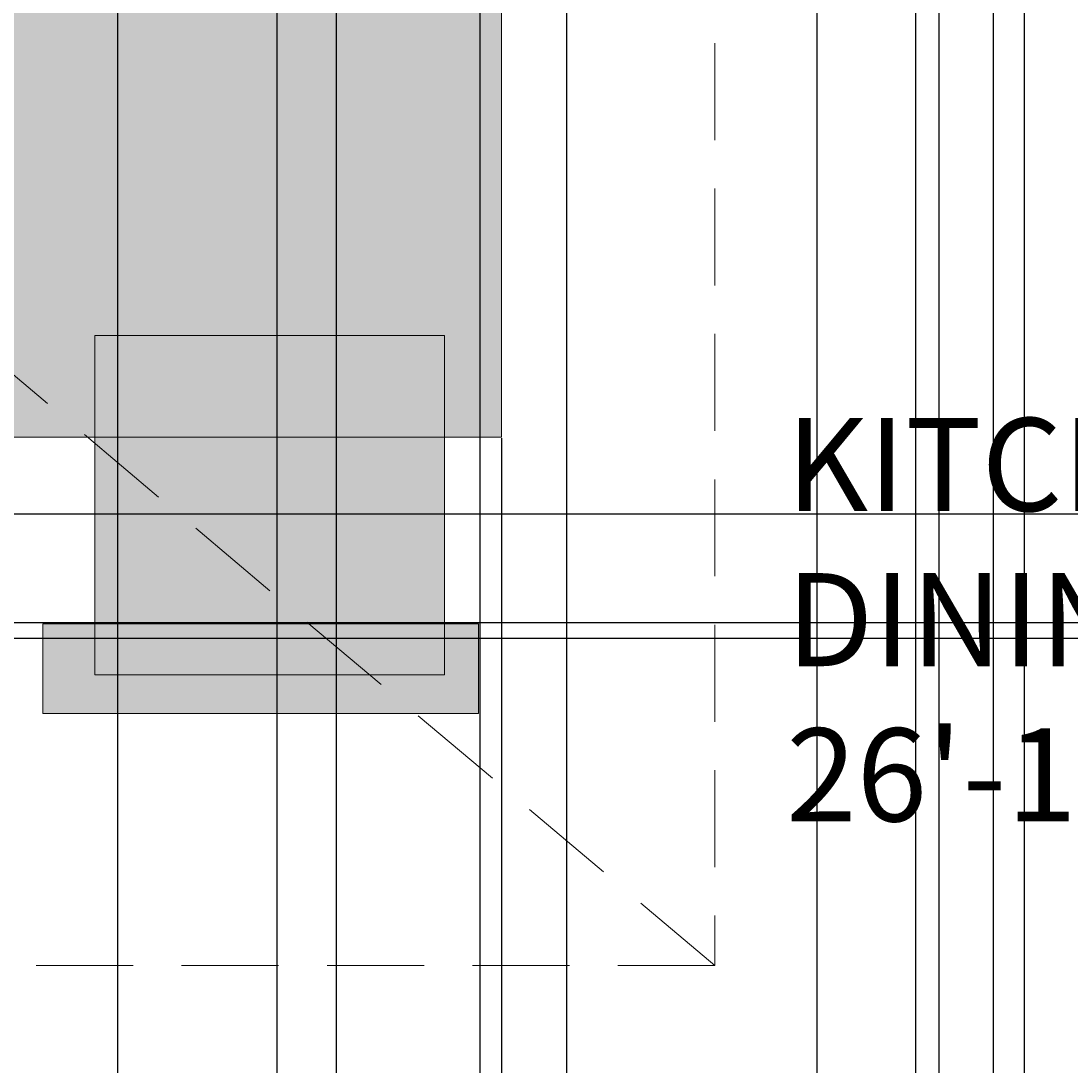
# Model space of a CAD drawing. Units: inches. Extents: x 818 to 1898, y 976 to 2364.
# Tile 71 of 96: x 1372 to 1439, y 1913 to 1980. Entities that reach past the tile are written whole.
import ezdxf

# ---------------------------------------------------------------- set-up
doc = ezdxf.new("R2010")
doc.units = ezdxf.units.IN
doc.header["$LTSCALE"] = 5
doc.header["$MEASUREMENT"] = 0
doc.linetypes.add('HIDDEN', pattern=[0.375, 0.25, -0.125])
for name, color, linetype, lineweight in [('A-ANNO-DIMS', 2, 'Continuous', 18), ('A-AREA-IDEN', 7, 'Continuous', 18), ('A-FLOR-OVHD', 8, 'HIDDEN', 13), ('A-FURN', 8, 'Continuous', 18), ('A-FURN-PATT', 8, 'Continuous', 9)]:
    doc.layers.add(name, color=color, linetype=linetype, lineweight=lineweight)
doc.styles.get("Standard").update_dxf_attribs({"font": 'arial.ttf'})
doc.dimstyles.get("Standard").update_dxf_attribs({"dimtxt": 0.18, "dimasz": 0.18, "dimexe": 0.18, "dimexo": 0.0625, "dimgap": 0.09, "dimtad": 0, "dimtih": 1, "dimtoh": 1, "dimdec": 4, "dimzin": 0, "dimdsep": 46, "dimtxsty": 'Standard', "dimcen": 0.09, "dimadec": 0, "dimazin": 0, "dimtfac": 1, "dimtdec": 4, "dimtofl": 0, "dimtmove": 0, "dimatfit": 3, "dimfxl": 1, "dimtolj": 1, "dimtzin": 0, "dimarcsym": 0})

# ---------------------------------------------------------------- blocks, each defined once
blk = doc.blocks.new('*D61')
at = {"layer": 'A-ANNO-DIMS', "color": 0, "lineweight": -2, "ltscale": 5, "transparency": 16777216}
for p, q in [((1071.725, 1203.027), (1071.725, 2363.873)), ((1071.905, 2363.693), (1250.936, 2363.693)), ((1430.545, 2363.693), (1251.514, 2363.693)), ((1430.725, 1203.027), (1430.725, 2363.873))]:
    blk.add_line(p, q, dxfattribs=at)
at = {"layer": 'A-ANNO-DIMS', "color": 0, "ltscale": 5, "transparency": 16777216}
for points in [[(1071.905, 2363.723), (1071.905, 2363.663), (1071.725, 2363.693)], [(1430.545, 2363.723), (1430.545, 2363.663), (1430.725, 2363.693)]]:
    blk.add_solid(points, dxfattribs=at)
at = {"layer": 'Defpoints', "color": 0, "ltscale": 5, "transparency": 16777216}
for p in [(1430.725, 2363.693), (1071.725, 1202.964), (1430.725, 1202.964)]:
    blk.add_point(p, dxfattribs=at)
at = {"layer": 'A-ANNO-DIMS', "color": 0, "ltscale": 5, "transparency": 16777216, "insert": (1251.225, 2363.693), "char_height": 0.18, "attachment_point": 5}
blk.add_mtext('\\A1;359', dxfattribs=at)
blk = doc.blocks.new('*D64')
at = {"layer": 'A-ANNO-DIMS', "color": 0, "lineweight": -2, "ltscale": 5, "transparency": 16777216}
for p, q in [((1197.725, 1501.141), (1197.725, 2363.873)), ((1197.905, 2363.693), (1313.935, 2363.693)), ((1430.545, 2363.693), (1314.516, 2363.693)), ((1430.725, 1501.141), (1430.725, 2363.873))]:
    blk.add_line(p, q, dxfattribs=at)
at = {"layer": 'A-ANNO-DIMS', "color": 0, "ltscale": 5, "transparency": 16777216}
for points in [[(1197.905, 2363.723), (1197.905, 2363.663), (1197.725, 2363.693)], [(1430.545, 2363.723), (1430.545, 2363.663), (1430.725, 2363.693)]]:
    blk.add_solid(points, dxfattribs=at)
at = {"layer": 'Defpoints', "color": 0, "ltscale": 5, "transparency": 16777216}
for p in [(1430.725, 2363.693), (1197.725, 1501.078), (1430.725, 1501.078)]:
    blk.add_point(p, dxfattribs=at)
at = {"layer": 'A-ANNO-DIMS', "color": 0, "ltscale": 5, "transparency": 16777216, "insert": (1314.225, 2363.693), "char_height": 0.18, "attachment_point": 5}
blk.add_mtext('\\A1;233', dxfattribs=at)
blk = doc.blocks.new('*D74')
at = {"layer": 'A-ANNO-DIMS', "color": 0, "lineweight": -2, "ltscale": 5, "transparency": 16777216}
for p, q in [((1590.663, 1940.078), (818.026, 1940.078)), ((818.206, 1939.898), (818.206, 1925.76)), ((818.206, 1911.258), (818.206, 1925.396)), ((1590.663, 1911.078), (818.026, 1911.078))]:
    blk.add_line(p, q, dxfattribs=at)
at = {"layer": 'A-ANNO-DIMS', "color": 0, "ltscale": 5, "transparency": 16777216}
for points in [[(818.176, 1939.898), (818.236, 1939.898), (818.206, 1940.078)], [(818.176, 1911.258), (818.236, 1911.258), (818.206, 1911.078)]]:
    blk.add_solid(points, dxfattribs=at)
at = {"layer": 'Defpoints', "color": 0, "ltscale": 5, "transparency": 16777216}
for p in [(818.206, 1940.078), (1590.725, 1940.078), (1590.725, 1911.078)]:
    blk.add_point(p, dxfattribs=at)
at = {"layer": 'A-ANNO-DIMS', "color": 0, "ltscale": 5, "transparency": 16777216, "insert": (818.206, 1925.578), "char_height": 0.18, "attachment_point": 5}
blk.add_mtext('\\A1;29', dxfattribs=at)
blk = doc.blocks.new('*D85')
at = {"layer": 'A-ANNO-DIMS', "color": 0, "lineweight": -2, "ltscale": 5, "transparency": 16777216}
for p, q in [((1258.788, 2053.078), (1897.916, 2053.078)), ((1897.736, 2052.898), (1897.736, 1876.76)), ((1897.736, 1700.258), (1897.736, 1876.396)), ((1258.788, 1700.078), (1897.916, 1700.078))]:
    blk.add_line(p, q, dxfattribs=at)
at = {"layer": 'A-ANNO-DIMS', "color": 0, "ltscale": 5, "transparency": 16777216}
for points in [[(1897.706, 2052.898), (1897.766, 2052.898), (1897.736, 2053.078)], [(1897.706, 1700.258), (1897.766, 1700.258), (1897.736, 1700.078)]]:
    blk.add_solid(points, dxfattribs=at)
at = {"layer": 'Defpoints', "color": 0, "ltscale": 5, "transparency": 16777216}
for p in [(1258.725, 2053.078), (1897.736, 2053.078), (1258.725, 1700.078)]:
    blk.add_point(p, dxfattribs=at)
at = {"layer": 'A-ANNO-DIMS', "color": 0, "ltscale": 5, "transparency": 16777216, "insert": (1897.736, 1876.578), "char_height": 0.18, "attachment_point": 5}
blk.add_mtext('\\A1;353', dxfattribs=at)
blk = doc.blocks.new('*D98')
at = {"layer": 'A-ANNO-DIMS', "color": 0, "lineweight": -2, "ltscale": 5, "transparency": 16777216}
for p, q in [((1338.541, 1071.118), (1338.541, 2363.873)), ((1338.721, 2363.693), (1364.815, 2363.693)), ((1391.696, 2363.693), (1365.602, 2363.693)), ((1391.876, 1071.118), (1391.876, 2363.873))]:
    blk.add_line(p, q, dxfattribs=at)
at = {"layer": 'A-ANNO-DIMS', "color": 0, "ltscale": 5, "transparency": 16777216}
for points in [[(1338.721, 2363.723), (1338.721, 2363.663), (1338.541, 2363.693)], [(1391.696, 2363.723), (1391.696, 2363.663), (1391.876, 2363.693)]]:
    blk.add_solid(points, dxfattribs=at)
at = {"layer": 'Defpoints', "color": 0, "ltscale": 5, "transparency": 16777216}
for p in [(1391.876, 2363.693), (1338.541, 1071.055), (1391.876, 1071.055)]:
    blk.add_point(p, dxfattribs=at)
at = {"layer": 'A-ANNO-DIMS', "color": 0, "ltscale": 5, "transparency": 16777216, "insert": (1365.208, 2363.693), "char_height": 0.18, "attachment_point": 5}
blk.add_mtext('\\A1;53.33', dxfattribs=at)
blk = doc.blocks.new('*D99')
at = {"layer": 'A-ANNO-DIMS', "color": 0, "lineweight": -2, "ltscale": 5, "transparency": 16777216}
for p, q in [((1391.876, 1071.118), (1391.876, 2363.873)), ((1392.056, 2363.693), (1420.454, 2363.693)), ((1449.64, 2363.693), (1421.241, 2363.693)), ((1449.82, 1071.118), (1449.82, 2363.873))]:
    blk.add_line(p, q, dxfattribs=at)
at = {"layer": 'A-ANNO-DIMS', "color": 0, "ltscale": 5, "transparency": 16777216}
for points in [[(1392.056, 2363.723), (1392.056, 2363.663), (1391.876, 2363.693)], [(1449.64, 2363.723), (1449.64, 2363.663), (1449.82, 2363.693)]]:
    blk.add_solid(points, dxfattribs=at)
at = {"layer": 'Defpoints', "color": 0, "ltscale": 5, "transparency": 16777216}
for p in [(1449.82, 2363.693), (1391.876, 1071.055), (1449.82, 1071.055)]:
    blk.add_point(p, dxfattribs=at)
at = {"layer": 'A-ANNO-DIMS', "color": 0, "ltscale": 5, "transparency": 16777216, "insert": (1420.848, 2363.693), "char_height": 0.18, "attachment_point": 5}
blk.add_mtext('\\A1;57.94', dxfattribs=at)
blk = doc.blocks.new('*D161')
at = {"layer": 'A-ANNO-DIMS', "color": 0, "lineweight": -2, "ltscale": 5, "transparency": 16777216}
for p, q in [((1429.225, 1876.141), (1429.225, 2363.873)), ((1429.405, 2363.693), (1509.589, 2363.693)), ((1590.545, 2363.693), (1510.361, 2363.693)), ((1590.725, 1876.141), (1590.725, 2363.873))]:
    blk.add_line(p, q, dxfattribs=at)
at = {"layer": 'A-ANNO-DIMS', "color": 0, "ltscale": 5, "transparency": 16777216}
for points in [[(1429.405, 2363.723), (1429.405, 2363.663), (1429.225, 2363.693)], [(1590.545, 2363.723), (1590.545, 2363.663), (1590.725, 2363.693)]]:
    blk.add_solid(points, dxfattribs=at)
at = {"layer": 'Defpoints', "color": 0, "ltscale": 5, "transparency": 16777216}
for p in [(1590.725, 2363.693), (1429.225, 1876.078), (1590.725, 1876.078)]:
    blk.add_point(p, dxfattribs=at)
at = {"layer": 'A-ANNO-DIMS', "color": 0, "ltscale": 5, "transparency": 16777216, "insert": (1509.975, 2363.693), "char_height": 0.18, "attachment_point": 5}
blk.add_mtext('\\A1;161.5', dxfattribs=at)
blk = doc.blocks.new('*D166')
at = {"layer": 'A-ANNO-DIMS', "color": 0, "lineweight": -2, "ltscale": 5, "transparency": 16777216}
for p, q in [((1401.146, 1510.141), (1401.146, 2363.873)), ((1401.326, 2363.693), (1415.54, 2363.693)), ((1430.545, 2363.693), (1416.331, 2363.693)), ((1430.725, 1510.141), (1430.725, 2363.873))]:
    blk.add_line(p, q, dxfattribs=at)
at = {"layer": 'A-ANNO-DIMS', "color": 0, "ltscale": 5, "transparency": 16777216}
for points in [[(1401.326, 2363.723), (1401.326, 2363.663), (1401.146, 2363.693)], [(1430.545, 2363.723), (1430.545, 2363.663), (1430.725, 2363.693)]]:
    blk.add_solid(points, dxfattribs=at)
at = {"layer": 'Defpoints', "color": 0, "ltscale": 5, "transparency": 16777216}
for p in [(1430.725, 2363.693), (1401.146, 1510.078), (1430.725, 1510.078)]:
    blk.add_point(p, dxfattribs=at)
at = {"layer": 'A-ANNO-DIMS', "color": 0, "ltscale": 5, "transparency": 16777216, "insert": (1415.936, 2363.693), "char_height": 0.18, "attachment_point": 5}
blk.add_mtext('\\A1;29.58', dxfattribs=at)
blk = doc.blocks.new('*D191')
at = {"layer": 'A-ANNO-DIMS', "color": 0, "lineweight": -2, "ltscale": 5, "transparency": 16777216}
for p, q in [((1434.225, 1409.115), (1434.225, 2363.873)), ((1434.405, 2363.693), (1435.076, 2363.693)), ((1436.045, 2363.693), (1435.375, 2363.693)), ((1436.225, 1409.115), (1436.225, 2363.873))]:
    blk.add_line(p, q, dxfattribs=at)
at = {"layer": 'A-ANNO-DIMS', "color": 0, "ltscale": 5, "transparency": 16777216}
for points in [[(1434.405, 2363.723), (1434.405, 2363.663), (1434.225, 2363.693)], [(1436.045, 2363.723), (1436.045, 2363.663), (1436.225, 2363.693)]]:
    blk.add_solid(points, dxfattribs=at)
at = {"layer": 'Defpoints', "color": 0, "ltscale": 5, "transparency": 16777216}
for p in [(1436.225, 2363.693), (1434.225, 1409.052), (1436.225, 1409.052)]:
    blk.add_point(p, dxfattribs=at)
at = {"layer": 'A-ANNO-DIMS', "color": 0, "ltscale": 5, "transparency": 16777216, "insert": (1435.225, 2363.693), "char_height": 0.18, "attachment_point": 5}
blk.add_mtext('\\A1;2', dxfattribs=at)
blk = doc.blocks.new('*D211')
at = {"layer": 'A-ANNO-DIMS', "color": 0, "lineweight": -2, "ltscale": 5, "transparency": 16777216}
for p, q in [((1599.66265, 1948.078237), (818.025912, 1948.078237)), ((818.205912, 1947.898237), (818.205912, 1944.758237)), ((818.205912, 1941.258237), (818.205912, 1944.398237)), ((1599.66265, 1941.078237), (818.025912, 1941.078237))]:
    blk.add_line(p, q, dxfattribs=at)
at = {"layer": 'A-ANNO-DIMS', "color": 0, "ltscale": 5, "transparency": 16777216}
for points in [[(818.175912, 1947.898237), (818.235912, 1947.898237), (818.205912, 1948.078237)], [(818.175912, 1941.258237), (818.235912, 1941.258237), (818.205912, 1941.078237)]]:
    blk.add_solid(points, dxfattribs=at)
at = {"layer": 'Defpoints', "color": 0, "ltscale": 5, "transparency": 16777216}
for p in [(818.205912, 1948.078237), (1599.72515, 1948.078237), (1599.72515, 1941.078237)]:
    blk.add_point(p, dxfattribs=at)
at = {"layer": 'A-ANNO-DIMS', "color": 0, "ltscale": 5, "transparency": 16777216, "insert": (818.205912, 1944.578237), "char_height": 0.18, "attachment_point": 5}
blk.add_mtext('\\A1;7', dxfattribs=at)
blk = doc.blocks.new('*D231')
at = {"layer": 'A-ANNO-DIMS', "color": 0, "lineweight": -2, "ltscale": 5, "transparency": 16777216}
for p, q in [((1303.931, 1952.978), (1303.931, 975.663)), ((1402.518, 1952.978), (1402.518, 975.663)), ((1304.111, 975.843), (1352.831, 975.843)), ((1402.338, 975.843), (1353.619, 975.843))]:
    blk.add_line(p, q, dxfattribs=at)
at = {"layer": 'A-ANNO-DIMS', "color": 0, "ltscale": 5, "transparency": 16777216}
for points in [[(1304.111, 975.873), (1304.111, 975.813), (1303.931, 975.843)], [(1402.338, 975.873), (1402.338, 975.813), (1402.518, 975.843)]]:
    blk.add_solid(points, dxfattribs=at)
at = {"layer": 'Defpoints', "color": 0, "ltscale": 5, "transparency": 16777216}
for p in [(1303.931, 1953.041), (1402.518, 1953.041), (1402.518, 975.843)]:
    blk.add_point(p, dxfattribs=at)
at = {"layer": 'A-ANNO-DIMS', "color": 0, "ltscale": 5, "transparency": 16777216, "insert": (1353.225, 975.843), "char_height": 0.18, "attachment_point": 5}
blk.add_mtext('\\A1;98.59', dxfattribs=at)
blk = doc.blocks.new('*D252')
at = {"layer": 'A-ANNO-DIMS', "color": 0, "lineweight": -2, "ltscale": 5, "transparency": 16777216}
for p, q in [((1330.305, 2053.016), (1330.305, 975.663)), ((1388.031, 2053.016), (1388.031, 975.663)), ((1330.485, 975.843), (1358.775, 975.843)), ((1387.851, 975.843), (1359.562, 975.843))]:
    blk.add_line(p, q, dxfattribs=at)
at = {"layer": 'A-ANNO-DIMS', "color": 0, "ltscale": 5, "transparency": 16777216}
for points in [[(1330.485, 975.873), (1330.485, 975.813), (1330.305, 975.843)], [(1387.851, 975.873), (1387.851, 975.813), (1388.031, 975.843)]]:
    blk.add_solid(points, dxfattribs=at)
at = {"layer": 'Defpoints', "color": 0, "ltscale": 5, "transparency": 16777216}
for p in [(1330.305, 2053.078), (1388.031, 2053.078), (1388.031, 975.843)]:
    blk.add_point(p, dxfattribs=at)
at = {"layer": 'A-ANNO-DIMS', "color": 0, "ltscale": 5, "transparency": 16777216, "insert": (1359.168, 975.843), "char_height": 0.18, "attachment_point": 5}
blk.add_mtext('\\A1;57.73', dxfattribs=at)
blk = doc.blocks.new('*D273')
at = {"layer": 'A-ANNO-DIMS', "color": 0, "lineweight": -2, "ltscale": 5, "transparency": 16777216}
for p, q in [((1406.725, 1587.479), (1406.725, 2363.873)), ((1406.905, 2363.693), (1418.505, 2363.693)), ((1430.545, 2363.693), (1418.945, 2363.693)), ((1430.725, 1587.479), (1430.725, 2363.873))]:
    blk.add_line(p, q, dxfattribs=at)
at = {"layer": 'A-ANNO-DIMS', "color": 0, "ltscale": 5, "transparency": 16777216}
for points in [[(1406.905, 2363.723), (1406.905, 2363.663), (1406.725, 2363.693)], [(1430.545, 2363.723), (1430.545, 2363.663), (1430.725, 2363.693)]]:
    blk.add_solid(points, dxfattribs=at)
at = {"layer": 'Defpoints', "color": 0, "ltscale": 5, "transparency": 16777216}
for p in [(1430.725, 2363.693), (1406.725, 1587.416), (1430.725, 1587.416)]:
    blk.add_point(p, dxfattribs=at)
at = {"layer": 'A-ANNO-DIMS', "color": 0, "ltscale": 5, "transparency": 16777216, "insert": (1418.725, 2363.693), "char_height": 0.18, "attachment_point": 5}
blk.add_mtext('\\A1;24', dxfattribs=at)
blk = doc.blocks.new('*D274')
at = {"layer": 'A-ANNO-DIMS', "color": 0, "lineweight": -2, "ltscale": 5, "transparency": 16777216}
for p, q in [((1311.025, 1897.929), (1311.025, 2363.873)), ((1311.205, 2363.693), (1344.007, 2363.693)), ((1377.599, 2363.693), (1344.797, 2363.693)), ((1377.779, 1897.929), (1377.779, 2363.873))]:
    blk.add_line(p, q, dxfattribs=at)
at = {"layer": 'A-ANNO-DIMS', "color": 0, "ltscale": 5, "transparency": 16777216}
for points in [[(1311.205, 2363.723), (1311.205, 2363.663), (1311.025, 2363.693)], [(1377.599, 2363.723), (1377.599, 2363.663), (1377.779, 2363.693)]]:
    blk.add_solid(points, dxfattribs=at)
at = {"layer": 'Defpoints', "color": 0, "ltscale": 5, "transparency": 16777216}
for p in [(1377.779, 2363.693), (1311.025, 1897.866), (1377.779, 1897.866)]:
    blk.add_point(p, dxfattribs=at)
at = {"layer": 'A-ANNO-DIMS', "color": 0, "ltscale": 5, "transparency": 16777216, "insert": (1344.402, 2363.693), "char_height": 0.18, "attachment_point": 5}
blk.add_mtext('\\A1;66.75', dxfattribs=at)
blk = doc.blocks.new('*D281')
at = {"layer": 'A-ANNO-DIMS', "color": 0, "lineweight": -2, "ltscale": 5, "transparency": 16777216}
for p, q in [((1250.303, 1913.703), (1250.303, 2363.873)), ((1250.483, 2363.693), (1420.121, 2363.693)), ((1590.545, 2363.693), (1420.907, 2363.693)), ((1590.725, 2011.141), (1590.725, 2363.873))]:
    blk.add_line(p, q, dxfattribs=at)
at = {"layer": 'A-ANNO-DIMS', "color": 0, "ltscale": 5, "transparency": 16777216}
for points in [[(1250.483, 2363.723), (1250.483, 2363.663), (1250.303, 2363.693)], [(1590.545, 2363.723), (1590.545, 2363.663), (1590.725, 2363.693)]]:
    blk.add_solid(points, dxfattribs=at)
at = {"layer": 'Defpoints', "color": 0, "ltscale": 5, "transparency": 16777216}
for p in [(1590.725, 2363.693), (1590.725, 2011.078), (1250.303, 1913.64)]:
    blk.add_point(p, dxfattribs=at)
at = {"layer": 'A-ANNO-DIMS', "color": 0, "ltscale": 5, "transparency": 16777216, "insert": (1420.514, 2363.693), "char_height": 0.18, "attachment_point": 5}
blk.add_mtext('\\A1;340.4', dxfattribs=at)
blk = doc.blocks.new('*D282')
at = {"layer": 'A-ANNO-DIMS', "color": 0, "lineweight": -2, "ltscale": 5, "transparency": 16777216}
for p, q in [((1422.083, 2081.188), (1897.916, 2081.188)), ((1897.736, 2081.008), (1897.736, 1884.315)), ((1897.736, 1687.258), (1897.736, 1883.951)), ((1463.788, 1687.078), (1897.916, 1687.078))]:
    blk.add_line(p, q, dxfattribs=at)
at = {"layer": 'A-ANNO-DIMS', "color": 0, "ltscale": 5, "transparency": 16777216}
for points in [[(1897.706, 2081.008), (1897.766, 2081.008), (1897.736, 2081.188)], [(1897.706, 1687.258), (1897.766, 1687.258), (1897.736, 1687.078)]]:
    blk.add_solid(points, dxfattribs=at)
at = {"layer": 'Defpoints', "color": 0, "ltscale": 5, "transparency": 16777216}
for p in [(1422.02, 2081.188), (1897.736, 2081.188), (1463.725, 1687.078)]:
    blk.add_point(p, dxfattribs=at)
at = {"layer": 'A-ANNO-DIMS', "color": 0, "ltscale": 5, "transparency": 16777216, "insert": (1897.736, 1884.133), "char_height": 0.18, "attachment_point": 5}
blk.add_mtext('\\A1;394.1', dxfattribs=at)
blk = doc.blocks.new('*D288')
at = {"layer": 'A-ANNO-DIMS', "color": 0, "lineweight": -2, "ltscale": 5, "transparency": 16777216}
for p, q in [((1422.876, 1742.674), (1422.876, 2363.873)), ((1423.056, 2363.693), (1466.906, 2363.693)), ((1511.545, 2363.693), (1467.695, 2363.693)), ((1511.725, 1716.108), (1511.725, 2363.873))]:
    blk.add_line(p, q, dxfattribs=at)
at = {"layer": 'A-ANNO-DIMS', "color": 0, "ltscale": 5, "transparency": 16777216}
for points in [[(1423.056, 2363.723), (1423.056, 2363.663), (1422.876, 2363.693)], [(1511.545, 2363.723), (1511.545, 2363.663), (1511.725, 2363.693)]]:
    blk.add_solid(points, dxfattribs=at)
at = {"layer": 'Defpoints', "color": 0, "ltscale": 5, "transparency": 16777216}
for p in [(1511.725, 2363.693), (1422.876, 1742.611), (1511.725, 1716.045)]:
    blk.add_point(p, dxfattribs=at)
at = {"layer": 'A-ANNO-DIMS', "color": 0, "ltscale": 5, "transparency": 16777216, "insert": (1467.3, 2363.693), "char_height": 0.18, "attachment_point": 5}
blk.add_mtext('\\A1;88.85', dxfattribs=at)

msp = doc.modelspace()

# ---------------------------------------------------------------- hatches: boundary and pattern name
at = {"layer": 'A-FURN-PATT', "ltscale": 5}
h = msp.add_hatch(color=256, dxfattribs=at)
h.dxf.hatch_style = 1
h.paths.add_polyline_path([(1341.9997, 1981.5338), (1317.9034, 2001.8247), (1314.2595, 2001.8247), (1314.2595, 2004.893), (1310.1046, 2008.3917), (1303.9314, 2008.3917), (1303.9314, 1953.0408), (1308.1629, 1953.0408), (1314.2595, 1958.1746), (1314.2595, 1959.6079), (1315.9616, 1959.6079)])
h.paths.add_polyline_path([(1341.9997, 1981.5338), (1315.9616, 1959.6079), (1336.7936, 1959.6079), (1336.7936, 1953.0408), (1345.3966, 1953.0408), (1345.3966, 1959.6079), (1368.0379, 1959.6079)])
h.paths.add_polyline_path([(1402.518, 2008.3917), (1398.8475, 2008.3917), (1398.8475, 2001.8247), (1376.3134, 2001.8247), (1376.3134, 2008.3917), (1373.8948, 2008.3917), (1367.9307, 2003.3695), (1367.9307, 2001.8247), (1366.0961, 2001.8247), (1341.9997, 1981.5338), (1368.0379, 1959.6079), (1375.8366, 1953.0408), (1376.3134, 1953.0408), (1376.3134, 1959.6079), (1398.8475, 1959.6079), (1398.8475, 1953.0408), (1402.518, 1953.0408)])
h.paths.add_polyline_path([(1366.0961, 2001.8247), (1345.3966, 2001.8247), (1345.3966, 2008.3917), (1336.7936, 2008.3917), (1336.7936, 2001.8247), (1317.9034, 2001.8247), (1341.9997, 1981.5338)])
h.paths.add_polyline_path([(1336.7936, 1959.6079), (1315.9616, 1959.6079), (1314.2595, 1958.1746), (1314.2595, 1953.0408), (1336.7936, 1953.0408)], flags=17)
h.paths.add_polyline_path([(1367.9307, 1959.6079), (1345.3966, 1959.6079), (1345.3966, 1953.0408), (1367.9307, 1953.0408)], flags=17)
h.paths.add_polyline_path([(1398.8475, 1959.6079), (1376.3134, 1959.6079), (1376.3134, 1953.0408), (1398.8475, 1953.0408)], flags=17)
h.paths.add_polyline_path([(1368.0379, 1959.6079), (1367.9307, 1959.6079), (1367.9307, 1953.0408), (1375.8366, 1953.0408)], flags=17)
h.paths.add_polyline_path([(1314.2595, 1958.1746), (1308.1629, 1953.0408), (1314.2595, 1953.0408)], flags=17)
h.paths.add_polyline_path([(1315.9616, 1959.6079), (1314.2595, 1959.6079), (1314.2595, 1958.1746)], flags=16)
h.paths.add_polyline_path([(1314.2595, 2008.3917), (1310.1046, 2008.3917), (1314.2595, 2004.893)], flags=17)
h.paths.add_polyline_path([(1336.7936, 2008.3917), (1314.2595, 2008.3917), (1314.2595, 2004.893), (1317.9034, 2001.8247), (1336.7936, 2001.8247)], flags=17)
h.paths.add_polyline_path([(1314.2595, 2004.893), (1314.2595, 2001.8247), (1317.9034, 2001.8247)], flags=16)
h.paths.add_polyline_path([(1367.9307, 2008.3917), (1345.3966, 2008.3917), (1345.3966, 2001.8247), (1366.0961, 2001.8247), (1367.9307, 2003.3695)], flags=17)
h.paths.add_polyline_path([(1398.8475, 2008.3917), (1376.3134, 2008.3917), (1376.3134, 2001.8247), (1398.8475, 2001.8247)], flags=17)
h.paths.add_polyline_path([(1373.8948, 2008.3917), (1367.9307, 2008.3917), (1367.9307, 2003.3695)], flags=17)
h.paths.add_polyline_path([(1367.9307, 2003.3695), (1366.0961, 2001.8247), (1367.9307, 2001.8247)], flags=16)
h.paths.add_polyline_path([(1546.1595, 2044.0782), (1451.7698, 2044.0782), (1451.7698, 2020.0782), (1546.1595, 2020.0782)])
h.paths.add_polyline_path([(1492.0729, 2040.001, 0.431429), (1491.8238, 2040.251), (1491.3087, 2040.251, 0.415217), (1491.0729, 2040.001)], flags=16)
h.paths.add_polyline_path([(1481.8346, 2039.6036), (1511.886, 2039.6036), (1511.886, 2024.9917), (1481.8346, 2024.9917)], flags=16)
h.paths.add_polyline_path([(1491.0729, 2039.4857), (1491.0729, 2039.501), (1492.0729, 2039.501, -0.4117484), (1491.8401, 2039.251), (1491.8229, 2039.251), (1491.8229, 2039.2509, 0.4325918), (1492.0729, 2039.501), (1491.0729, 2039.501, 0.432604), (1491.3229, 2039.2509), (1491.3229, 2039.251), (1491.325, 2039.251, -0.4165823)], flags=0)
h.paths.add_polyline_path([(1485.3701, 2030.9622), (1485.3701, 2034.3556, -0.4142136), (1488.3701, 2037.3556), (1490.3421, 2037.3556, -0.0779193), (1491.0729, 2038.751), (1495.0729, 2038.751, -0.3148679), (1496.07, 2037.1201, -0.3016609), (1497.9049, 2034.3556), (1497.9049, 2030.9622, -0.4142136), (1494.9049, 2027.9622), (1488.3701, 2027.9622, -0.4142136)], flags=0)
h.paths.add_polyline_path([(1490.3229, 2035.751, 0.2655648), (1491.3229, 2036.751), (1491.3229, 2037.126), (1491.0729, 2037.126, -0.7914183), (1490.5434, 2037.251, -0.7914183), (1491.0729, 2037.376), (1491.3229, 2037.376), (1491.3229, 2037.751), (1492.0729, 2037.751), (1492.0729, 2037.376), (1492.3229, 2037.376, -0.7914183), (1492.8524, 2037.251, -0.7914183), (1492.3229, 2037.126), (1492.1491, 2037.126, -0.0866263), (1492.5376, 2036.0294, 0.1070481), (1493.0729, 2035.751), (1490.3229, 2035.751)], flags=0)
h.paths.add_polyline_path([(1491.9774, 2037.251, -1), (1491.4184, 2037.251, -1)], flags=0)
h.paths.add_polyline_path([(1500.0743, 2028.6045), (1500.0743, 2029.4074), (1510.8414, 2029.4074), (1510.8414, 2028.6045)], flags=0)
h.paths.add_polyline_path([(1500.0743, 2030.5314), (1500.0743, 2031.3342), (1510.8414, 2031.3342), (1510.8414, 2030.5314)], flags=0)
h.paths.add_polyline_path([(1500.0743, 2032.94), (1500.0743, 2033.7428), (1510.8414, 2033.7428), (1510.8414, 2032.94)], flags=0)
h.paths.add_polyline_path([(1500.0743, 2035.7499), (1500.0743, 2036.5528), (1510.8414, 2036.5528), (1510.8414, 2035.7499)], flags=0)
h.paths.add_polyline_path([(1590.7251, 2044.0782), (1576.1595, 2044.0782), (1576.1595, 2020.0782), (1590.7251, 2020.0782)])
h.paths.add_polyline_path([(1668.4429, 2044.0782), (1599.7251, 2044.0782), (1599.7251, 2020.0782), (1668.4429, 2020.0782)])
h.paths.add_polyline_path([(1621.2588, 2040.001, 0.431429), (1621.0097, 2040.251), (1620.4946, 2040.251, 0.415217), (1620.2588, 2040.001)], flags=16)
h.paths.add_polyline_path([(1611.0205, 2024.9917), (1611.0205, 2039.6036), (1641.0719, 2039.6036), (1641.0719, 2024.9917)], flags=16)
h.paths.add_polyline_path([(1620.2588, 2039.4857), (1620.2588, 2039.501), (1621.2588, 2039.501, -0.4117484), (1621.026, 2039.251), (1621.0088, 2039.251), (1621.0088, 2039.2509, 0.4325918), (1621.2588, 2039.501), (1620.2588, 2039.501, 0.432604), (1620.5088, 2039.2509), (1620.5088, 2039.251), (1620.5109, 2039.251, -0.4165823)], flags=0)
h.paths.add_polyline_path([(1614.556, 2030.9622), (1614.556, 2034.3556, -0.4142136), (1617.556, 2037.3556), (1619.528, 2037.3556, -0.0779193), (1620.2588, 2038.751), (1624.2588, 2038.751, -0.3148679), (1625.2559, 2037.1201, -0.3016609), (1627.0908, 2034.3556), (1627.0908, 2030.9622, -0.4142136), (1624.0908, 2027.9622), (1617.556, 2027.9622, -0.4142136)], flags=0)
h.paths.add_polyline_path([(1619.5088, 2035.751, 0.2655648), (1620.5088, 2036.751), (1620.5088, 2037.126), (1620.2588, 2037.126, -0.7914183), (1619.7293, 2037.251, -0.7914183), (1620.2588, 2037.376), (1620.5088, 2037.376), (1620.5088, 2037.751), (1621.2588, 2037.751), (1621.2588, 2037.376), (1621.5088, 2037.376, -0.7914183), (1622.0383, 2037.251, -0.7914183), (1621.5088, 2037.126), (1621.335, 2037.126, -0.0866263), (1621.7235, 2036.0294, 0.1070481), (1622.2588, 2035.751), (1619.5088, 2035.751)], flags=0)
h.paths.add_polyline_path([(1620.6043, 2037.251, -1), (1621.1633, 2037.251, -1)], flags=0)
h.paths.add_polyline_path([(1629.2602, 2028.6045), (1629.2602, 2029.4074), (1640.0273, 2029.4074), (1640.0273, 2028.6045)], flags=0)
h.paths.add_polyline_path([(1629.2602, 2030.5314), (1629.2602, 2031.3342), (1640.0273, 2031.3342), (1640.0273, 2030.5314)], flags=0)
h.paths.add_polyline_path([(1629.2602, 2032.94), (1629.2602, 2033.7428), (1640.0273, 2033.7428), (1640.0273, 2032.94)], flags=0)
h.paths.add_polyline_path([(1629.2602, 2035.7499), (1629.2602, 2036.5528), (1640.0273, 2036.5528), (1640.0273, 2035.7499)], flags=0)
h.paths.add_polyline_path([(1705.7252, 2044.0782), (1698.4429, 2044.0782), (1698.4429, 2020.0782), (1705.7252, 2020.0782)])
h.paths.add_polyline_path([(1705.7252, 1972.0782), (1599.7251, 1972.0782), (1599.7251, 1948.0782), (1705.7252, 1948.0782)])
h.paths.add_polyline_path([(1550.0109, 1979.2444), (1483.5451, 1979.2444), (1483.5451, 1948.6602), (1550.0109, 1948.6602)])
h.paths.add_polyline_path([(1490.2586, 1948.6602), (1488.2586, 1948.6602), (1488.2586, 1941.1742, 0.4142136), (1491.2586, 1938.1742), (1500.7446, 1938.1742, -0.4142136)])
h.paths.add_polyline_path([(1513.2306, 1941.1742), (1513.2306, 1948.6602), (1511.2306, 1948.6602, -0.4142136), (1500.7446, 1938.1742), (1510.2306, 1938.1742, 0.4142136)])
h.paths.add_polyline_path([(1518.778, 1948.6602), (1516.778, 1948.6602), (1516.778, 1941.1742, 0.4142136), (1519.778, 1938.1742), (1529.264, 1938.1742, -0.4142136)])
h.paths.add_polyline_path([(1541.75, 1941.1742), (1541.75, 1948.6602), (1539.75, 1948.6602, -0.4142136), (1529.264, 1938.1742), (1538.75, 1938.1742, 0.4142136)])
h.paths.add_polyline_path([(1590.7251, 1900.0782), (1519.6413, 1900.0782), (1519.6413, 1876.0782), (1590.7251, 1876.0782)])
h = msp.add_hatch(color=256, dxfattribs=at)
h.dxf.hatch_style = 1
h.paths.add_polyline_path([(1336.7936, 1953.0408), (1314.2595, 1953.0408), (1314.2595, 1941.0096), (1336.7936, 1941.0096)])
h.paths.add_polyline_path([(1338.9915, 1941.0096), (1336.7936, 1941.0096), (1336.7936, 1937.7177), (1314.2595, 1937.7177), (1314.2595, 1941.0096), (1310.9077, 1941.0096), (1310.9077, 1935.2252), (1338.9915, 1935.2252)])
h.paths.add_polyline_path([(1336.7936, 1941.0096), (1314.2595, 1941.0096), (1314.2595, 1937.7177), (1336.7936, 1937.7177)], flags=17)
h.paths.add_polyline_path([(1367.9307, 1959.6079), (1345.3966, 1959.6079), (1345.3966, 1941.0096), (1367.9307, 1941.0096)])
h.paths.add_polyline_path([(1398.8475, 1953.0408), (1376.3134, 1953.0408), (1376.3134, 1952.6393), (1390.1242, 1941.0096), (1398.8475, 1941.0096)])
h.paths.add_polyline_path([(1376.3134, 1952.6393), (1376.3134, 1941.0096), (1390.1242, 1941.0096)], flags=17)
h.paths.add_polyline_path([(1370.1286, 1941.0096), (1367.9307, 1941.0096), (1367.9307, 1937.7177), (1345.3966, 1937.7177), (1345.3966, 1941.0096), (1342.0448, 1941.0096), (1342.0448, 1935.2252), (1370.1286, 1935.2252)])
h.paths.add_polyline_path([(1367.9307, 1941.0096), (1345.3966, 1941.0096), (1345.3966, 1937.7177), (1367.9307, 1937.7177)], flags=17)
h.paths.add_polyline_path([(1390.1242, 1941.0096), (1376.3134, 1941.0096), (1376.3134, 1937.7177), (1394.0336, 1937.7177)], flags=17)
h.paths.add_polyline_path([(1394.0336, 1937.7177), (1376.3134, 1937.7177), (1376.3134, 1941.0096), (1372.9616, 1941.0096), (1372.9616, 1935.2252), (1396.9935, 1935.2252)])
h.paths.add_polyline_path([(1398.8475, 1941.0096), (1390.1242, 1941.0096), (1394.0336, 1937.7177), (1398.8475, 1937.7177)])
h.paths.add_polyline_path([(1401.0455, 1941.0096), (1398.8475, 1941.0096), (1398.8475, 1937.7177), (1394.0336, 1937.7177), (1396.9935, 1935.2252), (1401.0455, 1935.2252)])
h.paths.add_polyline_path([(1336.7936, 2020.4229), (1314.2595, 2020.4229), (1314.2595, 2008.3917), (1336.7936, 2008.3917)])
h.paths.add_polyline_path([(1336.7936, 2023.7149), (1314.2595, 2023.7149), (1314.2595, 2020.4229), (1336.7936, 2020.4229)], flags=17)
h.paths.add_polyline_path([(1338.9915, 2026.2074), (1310.9077, 2026.2074), (1310.9077, 2020.4229), (1314.2595, 2020.4229), (1314.2595, 2023.7149), (1336.7936, 2023.7149), (1336.7936, 2020.4229), (1338.9915, 2020.4229)])
h.paths.add_polyline_path([(1367.9307, 2023.7149), (1345.3966, 2023.7149), (1345.3966, 2020.4229), (1367.9307, 2020.4229)], flags=17)
h.paths.add_polyline_path([(1370.1286, 2026.2074), (1342.0448, 2026.2074), (1342.0448, 2020.4229), (1345.3966, 2020.4229), (1345.3966, 2023.7149), (1367.9307, 2023.7149), (1367.9307, 2020.4229), (1370.1286, 2020.4229)])
h.paths.add_polyline_path([(1367.9307, 2020.4229), (1345.3966, 2020.4229), (1345.3966, 2008.3917), (1367.9307, 2008.3917)])
h.paths.add_polyline_path([(1398.8475, 2020.4229), (1388.1824, 2020.4229), (1376.3134, 2010.4284), (1376.3134, 2008.3917), (1398.8475, 2008.3917)])
h.paths.add_polyline_path([(1392.0918, 2023.7149), (1376.3134, 2023.7149), (1376.3134, 2020.4229), (1388.1824, 2020.4229)], flags=17)
h.paths.add_polyline_path([(1388.1824, 2020.4229), (1376.3134, 2020.4229), (1376.3134, 2010.4284)], flags=17)
h.paths.add_polyline_path([(1395.0518, 2026.2074), (1372.9616, 2026.2074), (1372.9616, 2020.4229), (1376.3134, 2020.4229), (1376.3134, 2023.7149), (1392.0918, 2023.7149)])
h.paths.add_polyline_path([(1398.8475, 2023.7149), (1392.0918, 2023.7149), (1388.1824, 2020.4229), (1398.8475, 2020.4229)])
h.paths.add_polyline_path([(1401.0455, 2026.2074), (1395.0518, 2026.2074), (1392.0918, 2023.7149), (1398.8475, 2023.7149), (1398.8475, 2020.4229), (1401.0455, 2020.4229)])
h.paths.add_polyline_path([(1327.0339, 1897.8663), (1311.025, 1897.8663), (1311.025, 1876.0782), (1327.0339, 1876.0782)])
h.paths.add_polyline_path([(1377.7791, 1897.8663), (1359.9579, 1897.8663), (1359.9579, 1876.0782), (1377.7791, 1876.0782)])
h.paths.add_polyline_path([(1430.7251, 1541.0439), (1406.7251, 1541.0439), (1406.7251, 1525.9965), (1430.7251, 1525.9965)])
h.paths.add_polyline_path([(1430.7251, 1587.4164), (1406.7251, 1587.4164), (1406.7251, 1570.9187), (1430.7251, 1570.9187)])

# ---------------------------------------------------------------- linework, layer by layer
at = {"layer": 'A-FLOR-OVHD', "ltscale": 5}
msp.add_line((1416.2743, 1918.9894), (1267.7252, 2044.0782), dxfattribs=at)
msp.add_lwpolyline([(1267.7252, 2044.0782), (1416.2743, 2044.0782), (1416.2743, 1918.9894), (1267.7252, 1918.9894)], close=True, dxfattribs=at)
at = {"layer": 'A-FURN'}
for points in [[(1303.9314, 2008.3917), (1402.518, 2008.3917), (1402.518, 1953.0408), (1303.9314, 1953.0408)], [(1376.3134, 1959.6079), (1398.8475, 1959.6079), (1398.8475, 1937.7177), (1376.3134, 1937.7177)], [(1372.9616, 1941.0096), (1401.0455, 1941.0096), (1401.0455, 1935.2252), (1372.9616, 1935.2252)]]:
    msp.add_lwpolyline(points, close=True, dxfattribs=at)

# ---------------------------------------------------------------- texts
at = {"layer": 'A-AREA-IDEN', "ltscale": 5, "insert": (1420.8692, 1954.2828), "char_height": 6, "attachment_point": 1}
msp.add_mtext_dynamic_manual_height_columns('KITCHEN/\\PDINING\\P26\'-11" X 14\'-0"', width=118.992422, gutter_width=1, heights=[0], dxfattribs=at)

# ---------------------------------------------------------------- dimensions: what is measured, and where the dimension line sits
at = {"layer": 'A-ANNO-DIMS', "ltscale": 5}
for base, p1, p2, override, picture, middle in [((1430.7251, 2363.6929), (1071.7251, 1202.9642), (1430.7251, 1202.9642), {"dimdec": 0, "dimlfac": 1, "dimrnd": 0, "dimzin": 0, "dimdsep": 46, "dimlunit": 2}, '*D61', (1251.2251, 2363.6929)), ((1430.7251, 2363.6929), (1197.7251, 1501.0782), (1430.7251, 1501.0782), {"dimdec": 0, "dimlfac": 1, "dimrnd": 0, "dimzin": 0, "dimdsep": 46, "dimlunit": 2}, '*D64', (1314.2251, 2363.6929)), ((1590.7251, 2363.6929), (1250.3029, 1913.6401), (1590.7251, 2011.0782), {"dimdec": 1, "dimlfac": 1, "dimrnd": 0, "dimzin": 0, "dimdsep": 46, "dimlunit": 2}, '*D281', (1420.514, 2363.6929)), ((1377.7791, 2363.6929), (1311.025, 1897.8663), (1377.7791, 1897.8663), {"dimdec": 2, "dimlfac": 1, "dimrnd": 0, "dimzin": 0, "dimdsep": 46, "dimlunit": 2}, '*D274', (1344.4021, 2363.6929)), ((1391.8757, 2363.6929), (1338.5412, 1071.0552), (1391.8757, 1071.0552), {"dimdec": 2, "dimlfac": 1, "dimrnd": 0, "dimzin": 0, "dimdsep": 46, "dimlunit": 2}, '*D98', (1365.2084, 2363.6929)), ((1449.8196, 2363.6929), (1391.8757, 1071.0552), (1449.8196, 1071.0552), {"dimdec": 2, "dimlfac": 1, "dimrnd": 0, "dimzin": 0, "dimdsep": 46, "dimlunit": 2}, '*D99', (1420.8477, 2363.6929)), ((1430.7251, 2363.6929), (1401.1463, 1510.0782), (1430.7251, 1510.0782), {"dimdec": 2, "dimlfac": 1, "dimrnd": 0, "dimzin": 0, "dimdsep": 46, "dimlunit": 2}, '*D166', (1415.9357, 2363.6929)), ((1430.7251, 2363.6929), (1406.7251, 1587.4164), (1430.7251, 1587.4164), {"dimdec": 0, "dimlfac": 1, "dimrnd": 0, "dimzin": 0, "dimdsep": 46, "dimlunit": 2}, '*D273', (1418.7251, 2363.6929)), ((1511.7251, 2363.6929), (1422.8756, 1742.6113), (1511.7251, 1716.0454), {"dimdec": 2, "dimlfac": 1, "dimrnd": 0, "dimzin": 0, "dimdsep": 46, "dimlunit": 2}, '*D288', (1467.3004, 2363.6929)), ((1590.7251, 2363.6929), (1429.2251, 1876.0782), (1590.7251, 1876.0782), {"dimdec": 1, "dimlfac": 1, "dimrnd": 0, "dimzin": 0, "dimdsep": 46, "dimlunit": 2}, '*D161', (1509.9751, 2363.6929)), ((1436.2251, 2363.6929), (1434.2251, 1409.0522), (1436.2251, 1409.0522), {"dimdec": 0, "dimlfac": 1, "dimrnd": 0, "dimzin": 0, "dimdsep": 46, "dimlunit": 2}, '*D191', (1435.2251, 2363.6929)), ((1388.0315, 975.8433), (1330.305, 2053.0782), (1388.0315, 2053.0782), {"dimdec": 2, "dimlfac": 1, "dimrnd": 0, "dimzin": 0, "dimdsep": 46, "dimlunit": 2}, '*D252', (1359.1682, 975.8433)), ((1402.518, 975.8433), (1303.9314, 1953.0408), (1402.518, 1953.0408), {"dimdec": 2, "dimlfac": 1, "dimrnd": 0, "dimzin": 0, "dimdsep": 46, "dimlunit": 2}, '*D231', (1353.2247, 975.8433))]:
    dim = msp.add_linear_dim(base=base, p1=p1, p2=p2, dimstyle='Standard', override=override, dxfattribs=at)
    dim.commit()
    dim.dimension.update_dxf_attribs({"geometry": picture, "text_midpoint": middle})
for base, p1, p2, override, picture, middle in [((1897.736, 2081.1881), (1463.7251, 1687.0782), (1422.02, 2081.1881), {"dimdec": 1, "dimlfac": 1, "dimrnd": 0, "dimzin": 0, "dimdsep": 46, "dimlunit": 2}, '*D282', (1897.736, 1884.1332)), ((1897.736, 2053.0782), (1258.7251, 1700.0782), (1258.7251, 2053.0782), {"dimdec": 0, "dimlfac": 1, "dimrnd": 0, "dimzin": 0, "dimdsep": 46, "dimlunit": 2}, '*D85', (1897.736, 1876.5782)), ((818.2059, 1948.0782), (1599.7251, 1941.0782), (1599.7251, 1948.0782), {"dimdec": 0, "dimlfac": 1, "dimrnd": 0, "dimzin": 0, "dimdsep": 46, "dimlunit": 2}, '*D211', (818.2059, 1944.5782)), ((818.2059, 1940.0782), (1590.7251, 1911.0782), (1590.7251, 1940.0782), {"dimdec": 0, "dimlfac": 1, "dimrnd": 0, "dimzin": 0, "dimdsep": 46, "dimlunit": 2}, '*D74', (818.2059, 1925.5782))]:
    dim = msp.add_linear_dim(base=base, p1=p1, p2=p2, angle=90, dimstyle='Standard', override=override, dxfattribs=at)
    dim.commit()
    dim.dimension.update_dxf_attribs({"geometry": picture, "text_midpoint": middle})

doc.saveas('drawing.dxf')
